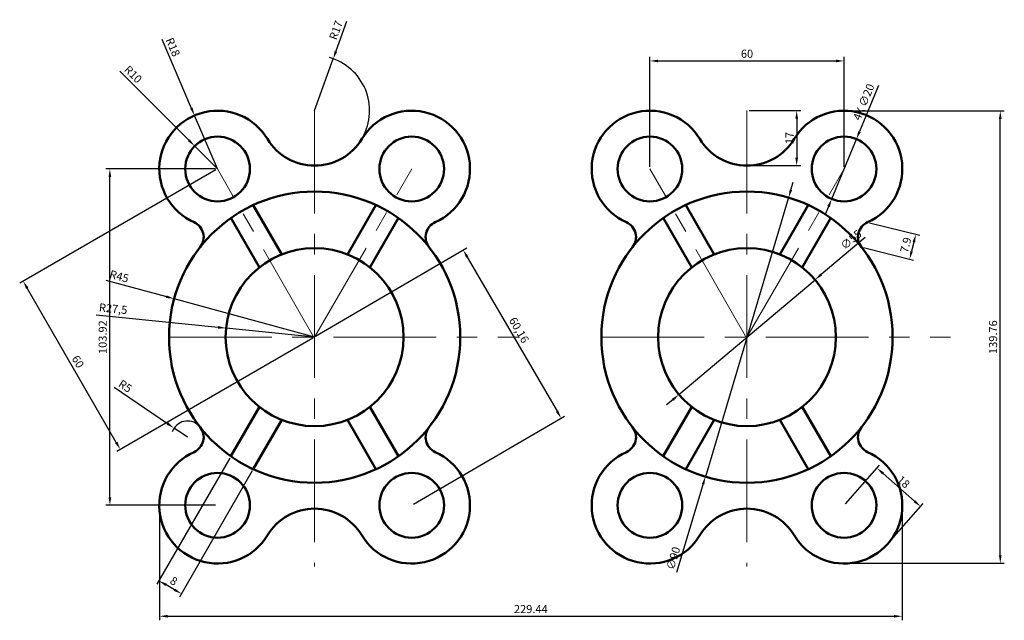
# Model space of a CAD drawing. Units: millimetres. Extents: x 2850 to 3154, y 1408 to 1594.
import ezdxf

# ---------------------------------------------------------------- set-up
doc = ezdxf.new("R2010")
doc.units = ezdxf.units.MM
doc.linetypes.add('CENTER', pattern=[50.8, 31.75, -6.35, 6.35, -6.35])
for name, color, linetype, lineweight in [('M-CNTR', 4, 'CENTER', 18), ('M-DIMS', 2, 'Continuous', 25), ('M-OUTL', 7, 'Continuous', 50)]:
    doc.layers.add(name, color=color, linetype=linetype, lineweight=lineweight)
doc.styles.get("Standard").update_dxf_attribs({"font": 'arial.ttf'})
doc.dimstyles.new('ISO-25', dxfattribs={"dimtxt": 2.5, "dimasz": 2.5, "dimexe": 1.25, "dimexo": 0.625, "dimtad": 1, "dimtxsty": 'Standard', "dimcen": 2.5, "dimadec": 0, "dimazin": 0, "dimtfac": 1, "dimtmove": 0, "dimatfit": 3, "dimfxl": 1, "dimarcsym": 0})

# ---------------------------------------------------------------- blocks, each defined once
blk = doc.blocks.new('*D1')
at = {"layer": 'Defpoints', "color": 0, "transparency": 16777216}
for p in [(2904.17, 1564.28), (2911.28, 1547.75)]:
    blk.add_point(p, dxfattribs=at)
at = {"layer": 'M-DIMS', "color": 0, "lineweight": -2, "transparency": 16777216}
for p, q in [((2894.02, 1587.85), (2903.18, 1566.58)), ((2911.28, 1547.75), (2904.17, 1564.28))]:
    blk.add_line(p, q, dxfattribs=at)
at = {"layer": 'M-DIMS', "color": 0, "transparency": 16777216}
blk.add_solid([(2903.56, 1566.74), (2902.79, 1566.42), (2904.17, 1564.28)], dxfattribs=at)
at = {"layer": 'M-DIMS', "color": 0, "transparency": 16777216, "insert": (2897.2, 1585.28), "char_height": 2.5, "attachment_point": 5, "rotation": 293.2898}
blk.add_mtext('R18', dxfattribs=at)
blk = doc.blocks.new('*D2')
at = {"layer": 'Defpoints', "color": 0, "transparency": 16777216}
for p in [(2904.22, 1554.83), (2911.28, 1547.75)]:
    blk.add_point(p, dxfattribs=at)
at = {"layer": 'M-DIMS', "color": 0, "lineweight": -2, "transparency": 16777216}
for p, q in [((2881.08, 1577.99), (2902.45, 1556.6)), ((2911.28, 1547.75), (2904.22, 1554.83))]:
    blk.add_line(p, q, dxfattribs=at)
at = {"layer": 'M-DIMS', "color": 0, "transparency": 16777216}
blk.add_solid([(2902.74, 1556.89), (2902.15, 1556.3), (2904.22, 1554.83)], dxfattribs=at)
at = {"layer": 'M-DIMS', "color": 0, "transparency": 16777216, "insert": (2884.98, 1576.78), "char_height": 2.5, "attachment_point": 5, "rotation": 314.9607}
blk.add_mtext('R10', dxfattribs=at)
blk = doc.blocks.new('*D3')
at = {"layer": 'Defpoints', "color": 0, "transparency": 16777216}
for p in [(2947.03, 1581.78), (2941.28, 1565.78)]:
    blk.add_point(p, dxfattribs=at)
at = {"layer": 'M-DIMS', "color": 0, "lineweight": -2, "transparency": 16777216}
for p, q in [((2951.16, 1593.28), (2947.87, 1584.13)), ((2941.28, 1565.78), (2947.03, 1581.78))]:
    blk.add_line(p, q, dxfattribs=at)
blk.add_arc((2941.28, 1565.78), 17, 331.1037, 74.4661, dxfattribs=at)
at = {"layer": 'M-DIMS', "color": 0, "transparency": 16777216}
blk.add_solid([(2947.48, 1584.27), (2948.26, 1583.99), (2947.03, 1581.78)], dxfattribs=at)
at = {"layer": 'M-DIMS', "color": 0, "transparency": 16777216, "insert": (2948.17, 1590.52), "char_height": 2.5, "attachment_point": 5, "rotation": 70.2532}
blk.add_mtext('R17', dxfattribs=at)
blk = doc.blocks.new('*D4')
at = {"layer": 'Defpoints', "color": 0, "transparency": 16777216}
for p in [(2897.86, 1467.68), (2901.99, 1464.87)]:
    blk.add_point(p, dxfattribs=at)
at = {"layer": 'M-DIMS', "color": 0, "lineweight": -2, "transparency": 16777216}
for p, q in [((2879.32, 1480.3), (2895.79, 1469.09)), ((2901.99, 1464.87), (2897.86, 1467.68))]:
    blk.add_line(p, q, dxfattribs=at)
blk.add_arc((2901.99, 1464.87), 5, 45.3642, 160.0799, dxfattribs=at)
at = {"layer": 'M-DIMS', "color": 0, "transparency": 16777216}
blk.add_solid([(2896.03, 1469.43), (2895.56, 1468.74), (2897.86, 1467.68)], dxfattribs=at)
at = {"layer": 'M-DIMS', "color": 0, "transparency": 16777216, "insert": (2882.58, 1480.38), "char_height": 2.5, "attachment_point": 5, "rotation": 325.756}
blk.add_mtext('R5', dxfattribs=at)
blk = doc.blocks.new('*D5')
at = {"layer": 'Defpoints', "color": 0, "transparency": 16777216}
for p in [(2897.87, 1507.64), (2941.28, 1495.79)]:
    blk.add_point(p, dxfattribs=at)
at = {"layer": 'M-DIMS', "color": 0, "lineweight": -2, "transparency": 16777216}
for p, q in [((2876.8, 1513.39), (2895.46, 1508.3)), ((2941.28, 1495.79), (2897.87, 1507.64))]:
    blk.add_line(p, q, dxfattribs=at)
at = {"layer": 'M-DIMS', "color": 0, "transparency": 16777216}
blk.add_solid([(2895.57, 1508.7), (2895.35, 1507.89), (2897.87, 1507.64)], dxfattribs=at)
at = {"layer": 'M-DIMS', "color": 0, "transparency": 16777216, "insert": (2880.8, 1514.26), "char_height": 2.5, "attachment_point": 5, "rotation": 344.7343}
blk.add_mtext('R45', dxfattribs=at)
blk = doc.blocks.new('*D6')
at = {"layer": 'Defpoints', "color": 0, "transparency": 16777216}
for p in [(2913.92, 1498.57), (2941.28, 1495.79)]:
    blk.add_point(p, dxfattribs=at)
at = {"layer": 'M-DIMS', "color": 0, "lineweight": -2, "transparency": 16777216}
for p, q in [((2873.73, 1502.65), (2911.44, 1498.82)), ((2941.28, 1495.79), (2913.92, 1498.57))]:
    blk.add_line(p, q, dxfattribs=at)
at = {"layer": 'M-DIMS', "color": 0, "transparency": 16777216}
blk.add_solid([(2911.48, 1499.23), (2911.39, 1498.4), (2913.92, 1498.57)], dxfattribs=at)
at = {"layer": 'M-DIMS', "color": 0, "transparency": 16777216, "insert": (2879, 1504.25), "char_height": 2.5, "attachment_point": 5, "rotation": 354.2028}
blk.add_mtext('R27,5', dxfattribs=at)
blk = doc.blocks.new('*D7')
at = {"layer": 'Defpoints', "color": 0, "transparency": 16777216}
for p in [(2915.41, 1458.97), (2922.34, 1454.97), (2893.2, 1420.5)]:
    blk.add_point(p, dxfattribs=at)
at = {"layer": 'M-DIMS', "color": 0, "lineweight": -2, "transparency": 16777216}
for p, q in [((2915.09, 1458.43), (2892.57, 1419.42)), ((2922.02, 1454.43), (2899.5, 1415.42)), ((2897.96, 1417.75), (2895.36, 1419.25))]:
    blk.add_line(p, q, dxfattribs=at)
at = {"layer": 'M-DIMS', "color": 0, "transparency": 16777216}
for points in [[(2895.57, 1419.61), (2895.15, 1418.89), (2893.2, 1420.5)], [(2898.17, 1418.11), (2897.75, 1417.39), (2900.12, 1416.5)]]:
    blk.add_solid(points, dxfattribs=at)
at = {"layer": 'M-DIMS', "color": 0, "transparency": 16777216, "insert": (2897.61, 1420.15), "char_height": 2.5, "attachment_point": 5, "rotation": 330}
blk.add_mtext('8', dxfattribs=at)
blk = doc.blocks.new('*D8')
at = {"layer": 'Defpoints', "color": 0, "transparency": 16777216}
for p in [(2941.01, 1495.82), (3017.46, 1470.72), (2971.28, 1443.83)]:
    blk.add_point(p, dxfattribs=at)
at = {"layer": 'M-DIMS', "color": 0, "lineweight": -2, "transparency": 16777216}
for p, q in [((2941.55, 1496.13), (2988.27, 1523.34)), ((2988.45, 1520.55), (3016.21, 1472.88)), ((2971.82, 1444.14), (3018.54, 1471.35))]:
    blk.add_line(p, q, dxfattribs=at)
at = {"layer": 'M-DIMS', "color": 0, "transparency": 16777216}
for points in [[(2988.81, 1520.76), (2988.09, 1520.34), (2987.19, 1522.71)], [(3016.57, 1473.09), (3015.85, 1472.67), (3017.46, 1470.72)]]:
    blk.add_solid(points, dxfattribs=at)
at = {"layer": 'M-DIMS', "color": 0, "transparency": 16777216, "insert": (3004.16, 1497.79), "char_height": 2.5, "attachment_point": 5, "rotation": 300.2133}
blk.add_mtext('60,16', dxfattribs=at)
blk = doc.blocks.new('*D9')
at = {"layer": 'Defpoints', "color": 0, "transparency": 16777216}
for p in [(2911.28, 1547.75), (2851.22, 1513.08), (2941.28, 1495.79)]:
    blk.add_point(p, dxfattribs=at)
at = {"layer": 'M-DIMS', "color": 0, "lineweight": -2, "transparency": 16777216}
for p, q in [((2910.74, 1547.44), (2850.14, 1512.45)), ((2879.97, 1463.28), (2852.47, 1510.91)), ((2940.74, 1495.48), (2880.14, 1460.49))]:
    blk.add_line(p, q, dxfattribs=at)
at = {"layer": 'M-DIMS', "color": 0, "transparency": 16777216}
for points in [[(2852.84, 1511.12), (2852.11, 1510.7), (2851.22, 1513.08)], [(2880.34, 1463.49), (2879.61, 1463.07), (2881.22, 1461.11)]]:
    blk.add_solid(points, dxfattribs=at)
at = {"layer": 'M-DIMS', "color": 0, "transparency": 16777216, "insert": (2867.87, 1488.05), "char_height": 2.5, "attachment_point": 5, "rotation": 300}
blk.add_mtext('60', dxfattribs=at)
blk = doc.blocks.new('HOUSING-FLANGED-4BOLT')
for p, q in [((-10.14, 25.56), (-18.95, 40.82)), ((10.14, 25.56), (18.95, 40.82)), ((-17.07, 21.56), (-25.88, 36.82)), ((17.07, 21.56), (25.88, 36.82)), ((-17.07, -21.56), (-25.88, -36.82)), ((17.07, -21.56), (25.88, -36.82)), ((-10.14, -25.56), (-18.95, -40.82)), ((10.14, -25.56), (18.95, -40.82))]:
    blk.add_line(p, q)
for points in [[(-35.36, 27.83, 0.489758), (-37.27, 35.5, -1.365948), (-14.57, 61.23, 0.565741), (14.57, 61.23, -1.365948), (37.27, 35.5, 0.489758), (35.36, 27.83)], [(35.36, -27.83, 0.489758), (37.27, -35.5, -1.365948), (14.57, -61.23, 0.565741), (-14.57, -61.23, -1.365948), (-37.27, -35.5, 0.489758), (-35.36, -27.83)]]:
    blk.add_lwpolyline(points, format="xyb")
for centre, radius in [((-30, 51.96), 10), ((30, 51.96), 10), ((0, 0), 45), ((0, 0), 27.5), ((-30, -51.96), 10), ((30, -51.96), 10)]:
    blk.add_circle(centre, radius)
blk = doc.blocks.new('*D11')
at = {"layer": 'Defpoints', "color": 0, "transparency": 16777216}
for p in [(3103.19, 1565.67), (3153.15, 1565.67), (3103.19, 1425.91)]:
    blk.add_point(p, dxfattribs=at)
at = {"layer": 'M-DIMS', "color": 0, "lineweight": -2, "transparency": 16777216}
for p, q in [((3103.82, 1565.67), (3154.4, 1565.67)), ((3153.15, 1428.41), (3153.15, 1563.17)), ((3103.82, 1425.91), (3154.4, 1425.91))]:
    blk.add_line(p, q, dxfattribs=at)
at = {"layer": 'M-DIMS', "color": 0, "transparency": 16777216}
for points in [[(3152.73, 1563.17), (3153.57, 1563.17), (3153.15, 1565.67)], [(3152.73, 1428.41), (3153.57, 1428.41), (3153.15, 1425.91)]]:
    blk.add_solid(points, dxfattribs=at)
at = {"layer": 'M-DIMS', "color": 0, "transparency": 16777216, "insert": (3151.25, 1495.79), "char_height": 2.5, "attachment_point": 5, "rotation": 90}
blk.add_mtext('139.76', dxfattribs=at)
blk = doc.blocks.new('*D12')
at = {"layer": 'Defpoints', "color": 0, "transparency": 16777216}
for p in [(2878.02, 1547.75), (2911.28, 1547.75), (2911.28, 1443.83)]:
    blk.add_point(p, dxfattribs=at)
at = {"layer": 'M-DIMS', "color": 0, "lineweight": -2, "transparency": 16777216}
for p, q in [((2910.66, 1547.75), (2876.77, 1547.75)), ((2878.02, 1446.33), (2878.02, 1545.25)), ((2910.66, 1443.83), (2876.77, 1443.83))]:
    blk.add_line(p, q, dxfattribs=at)
at = {"layer": 'M-DIMS', "color": 0, "transparency": 16777216}
for points in [[(2877.6, 1545.25), (2878.43, 1545.25), (2878.02, 1547.75)], [(2877.6, 1446.33), (2878.43, 1446.33), (2878.02, 1443.83)]]:
    blk.add_solid(points, dxfattribs=at)
at = {"layer": 'M-DIMS', "color": 0, "transparency": 16777216, "insert": (2876.11, 1495.79), "char_height": 2.5, "attachment_point": 5, "rotation": 90}
blk.add_mtext('103.92', dxfattribs=at)
blk = doc.blocks.new('*D13')
at = {"layer": 'Defpoints', "color": 0, "transparency": 16777216}
for p in [(3104.89, 1581.13), (3044.89, 1547.75), (3104.89, 1547.75)]:
    blk.add_point(p, dxfattribs=at)
at = {"layer": 'M-DIMS', "color": 0, "lineweight": -2, "transparency": 16777216}
for p, q in [((3044.89, 1548.38), (3044.89, 1582.38)), ((3104.89, 1548.38), (3104.89, 1582.38)), ((3047.39, 1581.13), (3102.39, 1581.13))]:
    blk.add_line(p, q, dxfattribs=at)
at = {"layer": 'M-DIMS', "color": 0, "transparency": 16777216}
for points in [[(3047.39, 1581.54), (3047.39, 1580.71), (3044.89, 1581.13)], [(3102.39, 1581.54), (3102.39, 1580.71), (3104.89, 1581.13)]]:
    blk.add_solid(points, dxfattribs=at)
at = {"layer": 'M-DIMS', "color": 0, "transparency": 16777216, "insert": (3074.89, 1583.03), "char_height": 2.5, "attachment_point": 5}
blk.add_mtext('60', dxfattribs=at)
blk = doc.blocks.new('*D14')
at = {"layer": 'Defpoints', "color": 0, "transparency": 16777216}
for p in [(2893.37, 1442.09), (3122.8, 1442.09), (3122.8, 1409.55)]:
    blk.add_point(p, dxfattribs=at)
at = {"layer": 'M-DIMS', "color": 0, "lineweight": -2, "transparency": 16777216}
for p, q in [((2893.37, 1441.46), (2893.37, 1408.3)), ((3122.8, 1441.46), (3122.8, 1408.3)), ((2895.87, 1409.55), (3120.3, 1409.55))]:
    blk.add_line(p, q, dxfattribs=at)
at = {"layer": 'M-DIMS', "color": 0, "transparency": 16777216}
for points in [[(2895.87, 1409.96), (2895.87, 1409.13), (2893.37, 1409.55)], [(3120.3, 1409.96), (3120.3, 1409.13), (3122.8, 1409.55)]]:
    blk.add_solid(points, dxfattribs=at)
at = {"layer": 'M-DIMS', "color": 0, "transparency": 16777216, "insert": (3008.09, 1411.45), "char_height": 2.5, "attachment_point": 5}
blk.add_mtext('229.44', dxfattribs=at)
blk = doc.blocks.new('*D15')
at = {"layer": 'Defpoints', "color": 0, "transparency": 16777216}
for p in [(3074.89, 1565.78), (3074.89, 1548.78), (3090.24, 1548.78)]:
    blk.add_point(p, dxfattribs=at)
at = {"layer": 'M-DIMS', "color": 0, "lineweight": -2, "transparency": 16777216}
for p, q in [((3075.51, 1565.78), (3091.49, 1565.78)), ((3090.24, 1563.28), (3090.24, 1551.28)), ((3075.51, 1548.78), (3091.49, 1548.78))]:
    blk.add_line(p, q, dxfattribs=at)
at = {"layer": 'M-DIMS', "color": 0, "transparency": 16777216}
for points in [[(3089.82, 1563.28), (3090.66, 1563.28), (3090.24, 1565.78)], [(3089.82, 1551.28), (3090.66, 1551.28), (3090.24, 1548.78)]]:
    blk.add_solid(points, dxfattribs=at)
at = {"layer": 'M-DIMS', "color": 0, "transparency": 16777216, "insert": (3088.36, 1557.28), "char_height": 2.5, "attachment_point": 5, "rotation": 90}
blk.add_mtext('17', dxfattribs=at)
blk = doc.blocks.new('*D16')
at = {"layer": 'Defpoints', "color": 0, "transparency": 16777216}
for p in [(3104.89, 1443.83), (3128.54, 1443.43), (3118.39, 1431.92)]:
    blk.add_point(p, dxfattribs=at)
at = {"layer": 'M-DIMS', "color": 0, "lineweight": -2, "transparency": 16777216}
for p, q in [((3105.3, 1444.3), (3115.87, 1456.28)), ((3116.92, 1453.69), (3126.67, 1445.09)), ((3118.8, 1432.39), (3129.37, 1444.37))]:
    blk.add_line(p, q, dxfattribs=at)
at = {"layer": 'M-DIMS', "color": 0, "transparency": 16777216}
for points in [[(3117.19, 1454), (3116.64, 1453.37), (3115.04, 1455.34)], [(3126.94, 1445.4), (3126.39, 1444.77), (3128.54, 1443.43)]]:
    blk.add_solid(points, dxfattribs=at)
at = {"layer": 'M-DIMS', "color": 0, "transparency": 16777216, "insert": (3123.05, 1450.81), "char_height": 2.5, "attachment_point": 5, "rotation": 318.5876}
blk.add_mtext('18', dxfattribs=at)
blk = doc.blocks.new('*D17')
at = {"layer": 'Defpoints', "color": 0, "transparency": 16777216}
for p in [(3112.16, 1531.28), (3110.25, 1523.62), (3125.15, 1519.91)]:
    blk.add_point(p, dxfattribs=at)
at = {"layer": 'M-DIMS', "color": 0, "lineweight": -2, "transparency": 16777216}
for p, q in [((3112.77, 1531.13), (3128.27, 1527.27)), ((3126.45, 1525.15), (3125.75, 1522.33)), ((3110.86, 1523.47), (3126.36, 1519.61))]:
    blk.add_line(p, q, dxfattribs=at)
at = {"layer": 'M-DIMS', "color": 0, "transparency": 16777216}
for points in [[(3126.05, 1525.25), (3126.86, 1525.05), (3127.06, 1527.57)], [(3125.35, 1522.44), (3126.15, 1522.23), (3125.15, 1519.91)]]:
    blk.add_solid(points, dxfattribs=at)
at = {"layer": 'M-DIMS', "color": 0, "transparency": 16777216, "insert": (3124.26, 1524.2), "char_height": 2.5, "attachment_point": 5, "rotation": 76.0149}
blk.add_mtext('7.9', dxfattribs=at)
blk = doc.blocks.new('*D18')
at = {"layer": 'Defpoints', "color": 0, "transparency": 16777216}
for p in [(3087.76, 1538.91), (3062.02, 1452.67)]:
    blk.add_point(p, dxfattribs=at)
at = {"layer": 'M-DIMS', "color": 0, "lineweight": -2, "transparency": 16777216}
for p, q in [((3088.47, 1541.31), (3089.19, 1543.7)), ((3087.76, 1538.91), (3062.02, 1452.67)), ((3053.22, 1423.18), (3061.31, 1450.27))]:
    blk.add_line(p, q, dxfattribs=at)
at = {"layer": 'M-DIMS', "color": 0, "transparency": 16777216}
for points in [[(3088.07, 1541.42), (3088.87, 1541.19), (3087.76, 1538.91)], [(3060.91, 1450.39), (3061.7, 1450.15), (3062.02, 1452.67)]]:
    blk.add_solid(points, dxfattribs=at)
at = {"layer": 'M-DIMS', "color": 0, "transparency": 16777216, "insert": (3052.41, 1427.36), "char_height": 2.5, "attachment_point": 5, "rotation": 73.3836}
blk.add_mtext('∅90', dxfattribs=at)
blk = doc.blocks.new('*D19')
at = {"layer": 'Defpoints', "color": 0, "transparency": 16777216}
for p in [(3095.91, 1513.52), (3053.87, 1478.06)]:
    blk.add_point(p, dxfattribs=at)
at = {"layer": 'M-DIMS', "color": 0, "lineweight": -2, "transparency": 16777216}
for p, q in [((3111.41, 1526.6), (3097.82, 1515.13)), ((3053.87, 1478.06), (3095.91, 1513.52)), ((3051.96, 1476.44), (3050.05, 1474.83))]:
    blk.add_line(p, q, dxfattribs=at)
at = {"layer": 'M-DIMS', "color": 0, "transparency": 16777216}
for points in [[(3097.55, 1515.45), (3098.09, 1514.82), (3095.91, 1513.52)], [(3051.69, 1476.76), (3052.23, 1476.13), (3053.87, 1478.06)]]:
    blk.add_solid(points, dxfattribs=at)
at = {"layer": 'M-DIMS', "color": 0, "transparency": 16777216, "insert": (3107.25, 1525.67), "char_height": 2.5, "attachment_point": 5, "rotation": 40.1535}
blk.add_mtext('∅55', dxfattribs=at)
blk = doc.blocks.new('*D20')
at = {"layer": 'Defpoints', "color": 0, "transparency": 16777216}
for p in [(3108.71, 1556.99), (3101.07, 1538.51)]:
    blk.add_point(p, dxfattribs=at)
at = {"layer": 'M-DIMS', "color": 0, "lineweight": -2, "transparency": 16777216}
for p, q in [((3115.53, 1573.52), (3109.66, 1559.3)), ((3101.07, 1538.51), (3108.71, 1556.99)), ((3100.12, 1536.2), (3099.16, 1533.89))]:
    blk.add_line(p, q, dxfattribs=at)
at = {"layer": 'M-DIMS', "color": 0, "transparency": 16777216}
for points in [[(3109.27, 1559.46), (3110.04, 1559.14), (3108.71, 1556.99)], [(3099.73, 1536.36), (3100.5, 1536.04), (3101.07, 1538.51)]]:
    blk.add_solid(points, dxfattribs=at)
at = {"layer": 'M-DIMS', "color": 0, "transparency": 16777216, "insert": (3111.25, 1568.32), "char_height": 2.5, "attachment_point": 5, "rotation": 67.5617}
blk.add_mtext('4X ∅20', dxfattribs=at)

msp = doc.modelspace()

# ---------------------------------------------------------------- linework, layer by layer
at = {"layer": 'M-CNTR'}
for p, q in [((2941.282, 1565.778), (2941.282, 1424.895)), ((3074.889, 1565.778), (3074.889, 1424.895)), ((2941.282, 1495.337), (2911.282, 1547.75)), ((2941.282, 1495.789), (2971.282, 1547.75)), ((3074.889, 1495.337), (3044.889, 1547.75)), ((3074.889, 1495.789), (3104.889, 1547.75)), ((2896.282, 1495.789), (3004.194, 1495.789)), ((3029.889, 1495.789), (3137.8, 1495.789))]:
    msp.add_line(p, q, dxfattribs=at)

# ---------------------------------------------------------------- block references
at = {"layer": 'M-OUTL'}
for p in [(2941.282, 1495.789), (3074.889, 1495.789)]:
    msp.add_blockref('HOUSING-FLANGED-4BOLT', p, dxfattribs=at)

# ---------------------------------------------------------------- dimensions: what is measured, and where the dimension line sits
at = {"layer": 'M-DIMS'}
dim = msp.add_radius_dim(center=(2941.282, 1565.778), mpoint=(2947.026, 1581.778), dimstyle='ISO-25', override={"dimclrd": 0, "dimclre": 0, "dimclrt": 0}, dxfattribs=at)
dim.commit()
dim.dimension.update_dxf_attribs({"geometry": '*D3', "text_midpoint": (2948.166, 1590.519)})
for center, mpoint, picture, middle in [((2911.282, 1547.75), (2904.165, 1564.284), '*D1', (2895.451, 1584.528)), ((2911.282, 1547.75), (2904.216, 1554.826), '*D2', (2883.63, 1575.441)), ((2941.282, 1495.789), (2897.87, 1507.637), '*D5', (2880.296, 1512.434)), ((2941.282, 1495.789), (2913.923, 1498.567), '*D6', (2878.78, 1502.134)), ((2901.991, 1464.867), (2897.857, 1467.681), '*D4', (2881.508, 1478.81))]:
    dim = msp.add_radius_dim(center=center, mpoint=mpoint, dimstyle='ISO-25', override={"dimclrd": 0, "dimclre": 0, "dimclrt": 0}, dxfattribs=at)
    dim.commit()
    dim.dimension.update_dxf_attribs({"geometry": picture, "text_midpoint": middle, "dimtype": 164})
for base, p1, p2, override, picture, middle in [((3104.889, 1581.128), (3044.889, 1547.75), (3104.889, 1547.75), {"dimdec": 0, "dimlfac": 1, "dimrnd": 0, "dimzin": 0, "dimdsep": 46, "dimlunit": 2}, '*D13', (3074.889, 1583.03)), ((3122.804, 1409.545), (2893.367, 1442.086), (3122.804, 1442.086), {"dimdec": 2, "dimlfac": 1, "dimrnd": 0, "dimzin": 0, "dimdsep": 46, "dimlunit": 2}, '*D14', (3008.085, 1411.447))]:
    dim = msp.add_linear_dim(base=base, p1=p1, p2=p2, dimstyle='ISO-25', override=override, dxfattribs=at)
    dim.commit()
    dim.dimension.update_dxf_attribs({"geometry": picture, "text_midpoint": middle})
dim = msp.add_diameter_dim_2p(p1=(3101.072, 1538.507), p2=(3108.705, 1556.993), text='4X <>', dimstyle='ISO-25', override={"dimdec": 0, "dimlfac": 1, "dimrnd": 0, "dimzin": 0, "dimdsep": 46, "dimlunit": 2}, dxfattribs=at)
dim.commit()
dim.dimension.update_dxf_attribs({"geometry": '*D20', "text_midpoint": (3113.072, 1567.568)})
for base, p1, p2, angle, override, picture, middle in [((3090.239, 1548.778), (3074.889, 1565.778), (3074.889, 1548.778), 270, {"dimdec": 0, "dimlfac": 1, "dimrnd": 0, "dimzin": 0, "dimdsep": 46, "dimlunit": 2}, '*D15', (3088.358, 1557.278)), ((3153.1503, 1565.6713), (3103.1902, 1425.9064), (3103.1902, 1565.6713), 90, {"dimdec": 2, "dimlfac": 1, "dimrnd": 0, "dimzin": 0, "dimdsep": 46, "dimlunit": 2}, '*D11', (3151.248, 1495.7888)), ((2878.017, 1547.75), (2911.282, 1443.827), (2911.282, 1547.75), 90, {"dimdec": 2, "dimlfac": 1, "dimrnd": 0, "dimzin": 0, "dimdsep": 46, "dimlunit": 2}, '*D12', (2876.114, 1495.789)), ((3125.146, 1519.909), (3112.16, 1531.285), (3110.251, 1523.619), 256.01488, {"dimdec": 1, "dimlfac": 1, "dimrnd": 0, "dimzin": 0, "dimdsep": 46, "dimlunit": 2}, '*D17', (3124.256, 1524.201)), ((3128.542, 1443.433), (3104.889, 1443.827), (3118.388, 1431.921), 318.58758, {"dimdec": 0, "dimlfac": 1, "dimrnd": 0, "dimzin": 0, "dimdsep": 46, "dimlunit": 2}, '*D16', (3123.05, 1450.812))]:
    dim = msp.add_linear_dim(base=base, p1=p1, p2=p2, angle=angle, dimstyle='ISO-25', override=override, dxfattribs=at)
    dim.commit()
    dim.dimension.update_dxf_attribs({"geometry": picture, "text_midpoint": middle})
for p1, p2, distance, picture, middle in [((2941.282, 1495.789), (2911.282, 1547.75), 69.349, '*D9', (2867.871, 1488.046)), ((2941.007, 1495.817), (2971.282, 1443.827), 53.441, '*D8', (3004.165, 1497.785)), ((2922.335, 1454.972), (2915.407, 1458.972), 44.423, '*D7', (2897.611, 1420.148))]:
    dim = msp.add_aligned_dim(p1=p1, p2=p2, distance=distance, dimstyle='ISO-25', override={"dimclrd": 0, "dimclre": 0, "dimclrt": 0}, dxfattribs=at)
    dim.commit()
    dim.dimension.update_dxf_attribs({"geometry": picture, "text_midpoint": middle})
for p1, p2, picture, middle in [((3087.757, 1538.91), (3062.02, 1452.668), '*D18', (3054.299, 1426.796)), ((3053.87, 1478.056), (3095.907, 1513.522), '*D19', (3108.519, 1524.162))]:
    dim = msp.add_diameter_dim_2p(p1=p1, p2=p2, dimstyle='ISO-25', override={"dimdec": 0, "dimlfac": 1, "dimrnd": 0, "dimzin": 0, "dimdsep": 46, "dimlunit": 2}, dxfattribs=at)
    dim.commit()
    dim.dimension.update_dxf_attribs({"geometry": picture, "text_midpoint": middle, "dimtype": 163})

doc.saveas('drawing.dxf')
